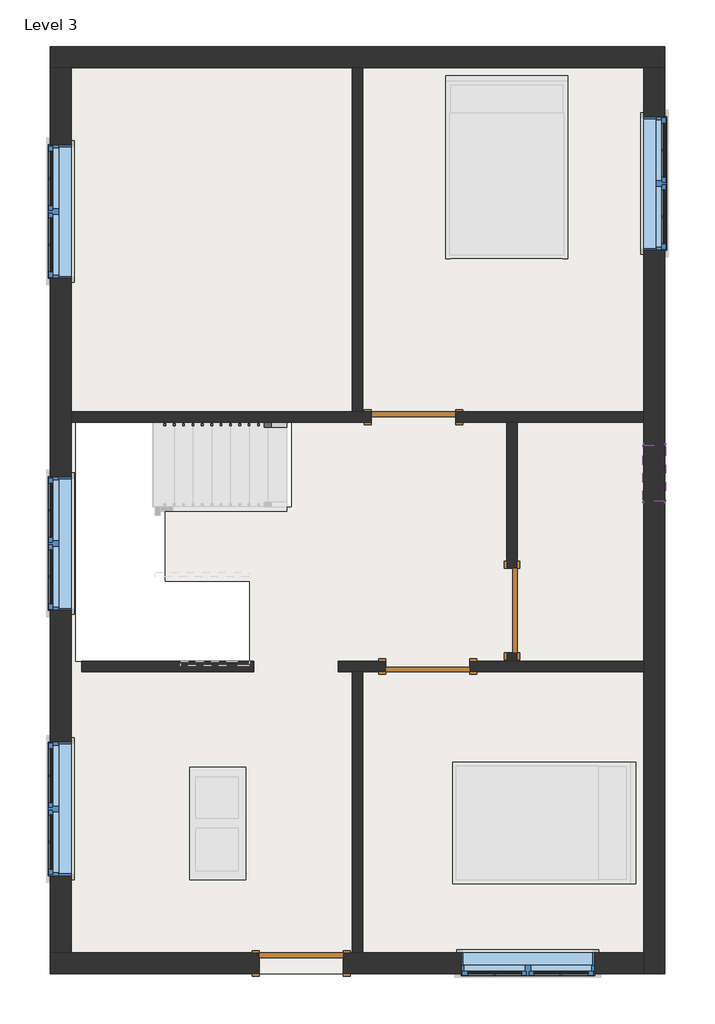
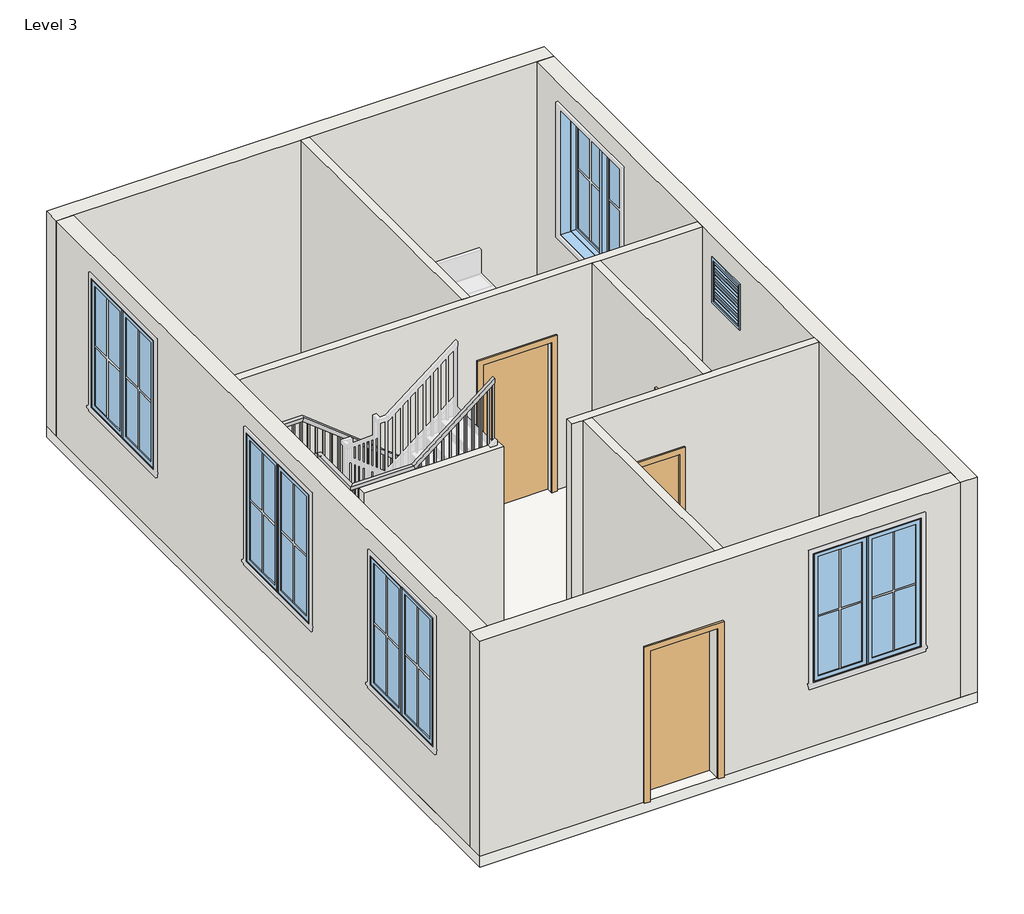
# One storey, part 1 of 2: 10 walls, 6 windows, 4 doors, 1 railing, 1 slab.
"""IFC4 building model written with IfcOpenShell, lengths in millimetres."""

from ifc_helpers import new_model, si_unit, frame, origin, place, context, project, spatial, polyline, outline, extrude, faceted_brep, transform, mapped, element, save
from components import door_e5f9f3c4, door_0ca8825f, window_9ac97e1a, window_f2d8fef0

model = new_model("IFC4")

# Units and contexts
model_context = context("Model", 3, world=origin())
ifc_project = project(units=[si_unit("LENGTHUNIT", "METRE", prefix="MILLI")], contexts=[model_context])

# Site, building, storey
site = spatial("IfcSite", under=ifc_project)
building = spatial("IfcBuilding", under=site)
storey = spatial("IfcBuildingStorey", under=building, Name="Level 3", Elevation=3200.4)

# Doors
placement = place(None, origin())
door_shape = door_e5f9f3c4(model_context)
element("IfcDoor", 1, ObjectType="Single-Flush : 36\" x 84\"", at=placement, inside=storey, context=model_context, shape_type="MappedRepresentation", body=[
    mapped(door_shape, transform((-2225.1840247, 979.1819954, 3200.4), x_axis=(1.0, 0.0, 0.0), y_axis=(0.0, 1.0, 0.0), z_axis=(0.0, 0.0, 1.0))),
])
element("IfcDoor", 2, ObjectType="Single-Flush : 36\" x 84\"", at=placement, inside=storey, context=model_context, shape_type="MappedRepresentation", body=[
    mapped(door_shape, transform((-1158.3840247, -1116.3180046, 3200.4), x_axis=(0.0, -1.0, 0.0), y_axis=(1.0, 0.0, 0.0), z_axis=(0.0, 0.0, 1.0))),
])
element("IfcDoor", 3, ObjectType="Single-Flush : 36\" x 84\"", at=placement, inside=storey, context=model_context, shape_type="MappedRepresentation", body=[
    mapped(door_shape, transform((-2072.7840247, -1725.9180046, 3200.4), x_axis=(-1.0, 0.0, 0.0), y_axis=(0.0, -1.0, 0.0), z_axis=(0.0, 0.0, 1.0))),
])
door_2_shape = door_0ca8825f(model_context)
element("IfcDoor", 4, ObjectType="Single-Flush : 36\" x 84\"", at=placement, inside=storey, context=model_context, shape_type="MappedRepresentation", body=[
    mapped(door_2_shape, transform((-3444.3840247, -4945.3680046, 3200.4), x_axis=(1.0, 0.0, 0.0), y_axis=(0.0, 1.0, 0.0), z_axis=(0.0, 0.0, 1.0))),
])

# Railing
element("IfcRailing", 5, ObjectType="Handrail - Rectangular", at=placement, inside=storey, context=model_context, shape_type="SolidModel", body=[
    faceted_brep([(-3603.1340247, 871.2319954, 4275.2210526), (-3603.1340247, 871.2319954, 4210.4980109), (-3603.1340247, 922.0319954, 4210.4980109), (-3603.1340247, 922.0319954, 4275.2210526), (-5097.5006913, 871.2319954, 5454.9842105), (-5115.1365442, 871.2319954, 5404.1842105), (-5115.1365442, 922.0319954, 5404.1842105), (-5097.5006913, 922.0319954, 5454.9842105), (-5889.1340247, 871.2319954, 5454.9842105), (-5889.1340247, 871.2319954, 5404.1842105), (-5939.9340247, 922.0319954, 5404.1842105), (-5939.9340247, 922.0319954, 5454.9842105), (-5889.1340247, 130.6632454, 5454.9842105), (-5889.1340247, 112.1228815, 5404.1842105), (-5939.9340247, 112.1228815, 5404.1842105), (-5939.9340247, 130.6632454, 5454.9842105), (-5889.1340247, -877.3992546, 6303.8789474), (-5889.1340247, -895.9396185, 6253.0789474), (-5939.9340247, -895.9396185, 6253.0789474), (-5939.9340247, -877.3992546, 6303.8789474), (-5889.1340247, -1617.9680046, 6303.8789474), (-5889.1340247, -1617.9680046, 6253.0789474), (-5939.9340247, -1668.7680046, 6253.0789474), (-5939.9340247, -1668.7680046, 6303.8789474), (-5097.5006913, -1617.9680046, 6303.8789474), (-5079.8648385, -1617.9680046, 6253.0789474), (-5079.8648385, -1668.7680046, 6253.0789474), (-5097.5006913, -1668.7680046, 6303.8789474), (-4009.5340247, -1617.9680046, 7162.8), (-4009.5340247, -1668.7680046, 7162.8), (-4009.5340247, -1668.7680046, 7098.0769583), (-4009.5340247, -1617.9680046, 7098.0769583)], [[[0, 1, 2, 3]], [[1, 0, 4, 5]], [[2, 1, 5, 6]], [[3, 2, 6, 7]], [[0, 3, 7, 4]], [[5, 4, 8, 9]], [[6, 5, 9, 10]], [[7, 6, 10, 11]], [[4, 7, 11, 8]], [[9, 8, 12, 13]], [[10, 9, 13, 14]], [[11, 10, 14, 15]], [[8, 11, 15, 12]], [[13, 12, 16, 17]], [[14, 13, 17, 18]], [[15, 14, 18, 19]], [[12, 15, 19, 16]], [[17, 16, 20, 21]], [[18, 17, 21, 22]], [[19, 18, 22, 23]], [[16, 19, 23, 20]], [[21, 20, 24, 25]], [[22, 21, 25, 26]], [[23, 22, 26, 27]], [[20, 23, 27, 24]], [[28, 29, 30, 31]], [[25, 24, 28, 31]], [[26, 25, 31, 30]], [[27, 26, 30, 29]], [[24, 27, 29, 28]]]),
    extrude(outline(polyline([(7045.4388004, -4076.2090247), (7030.3993267, -4095.2590247), (6087.9789474, -4095.2590247), (6087.9789474, -4076.2090247), (7045.4388004, -4076.2090247)])), frame((0.0, -1652.8930046, 0.0), z_axis=(0.0, 1.0, 0.0), x_axis=(0.0, 0.0, 1.0)), (0.0, 0.0, 1.0), 19.05),
    extrude(outline(polyline([(6965.228274, -4177.8090247), (6950.1888004, -4196.8590247), (6087.9789474, -4196.8590247), (6087.9789474, -4177.8090247), (6965.228274, -4177.8090247)])), frame((0.0, -1652.8930046, 0.0), z_axis=(0.0, 1.0, 0.0), x_axis=(0.0, 0.0, 1.0)), (0.0, 0.0, 1.0), 19.05),
    extrude(outline(polyline([(6885.0177477, -4279.4090247), (6869.978274, -4298.4590247), (5927.5578947, -4298.4590247), (5927.5578947, -4279.4090247), (6885.0177477, -4279.4090247)])), frame((0.0, -1652.8930046, 0.0), z_axis=(0.0, 1.0, 0.0), x_axis=(0.0, 0.0, 1.0)), (0.0, 0.0, 1.0), 19.05),
    extrude(outline(polyline([(6804.8072214, -4381.0090247), (6789.7677477, -4400.0590247), (5927.5578947, -4400.0590247), (5927.5578947, -4381.0090247), (6804.8072214, -4381.0090247)])), frame((0.0, -1652.8930046, 0.0), z_axis=(0.0, 1.0, 0.0), x_axis=(0.0, 0.0, 1.0)), (0.0, 0.0, 1.0), 19.05),
    extrude(outline(polyline([(6724.5966951, -4482.6090247), (6709.5572214, -4501.6590247), (5767.1368421, -4501.6590247), (5767.1368421, -4482.6090247), (6724.5966951, -4482.6090247)])), frame((0.0, -1652.8930046, 0.0), z_axis=(0.0, 1.0, 0.0), x_axis=(0.0, 0.0, 1.0)), (0.0, 0.0, 1.0), 19.05),
    extrude(outline(polyline([(6644.3861688, -4584.2090247), (6629.3466951, -4603.2590247), (5767.1368421, -4603.2590247), (5767.1368421, -4584.2090247), (6644.3861688, -4584.2090247)])), frame((0.0, -1652.8930046, 0.0), z_axis=(0.0, 1.0, 0.0), x_axis=(0.0, 0.0, 1.0)), (0.0, 0.0, 1.0), 19.05),
    extrude(outline(polyline([(6564.1756425, -4685.8090247), (6549.1361688, -4704.8590247), (5606.7157895, -4704.8590247), (5606.7157895, -4685.8090247), (6564.1756425, -4685.8090247)])), frame((0.0, -1652.8930046, 0.0), z_axis=(0.0, 1.0, 0.0), x_axis=(0.0, 0.0, 1.0)), (0.0, 0.0, 1.0), 19.05),
    extrude(outline(polyline([(6483.9651161, -4787.4090247), (6468.9256425, -4806.4590247), (5606.7157895, -4806.4590247), (5606.7157895, -4787.4090247), (6483.9651161, -4787.4090247)])), frame((0.0, -1652.8930046, 0.0), z_axis=(0.0, 1.0, 0.0), x_axis=(0.0, 0.0, 1.0)), (0.0, 0.0, 1.0), 19.05),
    extrude(outline(polyline([(6403.7545898, -4889.0090247), (6388.7151161, -4908.0590247), (5446.2947368, -4908.0590247), (5446.2947368, -4889.0090247), (6403.7545898, -4889.0090247)])), frame((0.0, -1652.8930046, 0.0), z_axis=(0.0, 1.0, 0.0), x_axis=(0.0, 0.0, 1.0)), (0.0, 0.0, 1.0), 19.05),
    extrude(outline(polyline([(6323.5440635, -4990.6090247), (6308.5045898, -5009.6590247), (5446.2947368, -5009.6590247), (5446.2947368, -4990.6090247), (6323.5440635, -4990.6090247)])), frame((0.0, -1652.8930046, 0.0), z_axis=(0.0, 1.0, 0.0), x_axis=(0.0, 0.0, 1.0)), (0.0, 0.0, 1.0), 19.05),
    extrude(outline(polyline([(-5111.2590247, -1652.8930046), (-5111.2590247, -1633.8430046), (-5092.2090247, -1633.8430046), (-5092.2090247, -1652.8930046), (-5111.2590247, -1652.8930046)])), frame((0.0, 0.0, 5285.8736842), z_axis=(0.0, 0.0, 1.0), x_axis=(1.0, 0.0, 0.0)), (0.0, 0.0, 1.0), 967.2052632),
    extrude(outline(polyline([(-5212.8590247, -1652.8930046), (-5212.8590247, -1633.8430046), (-5193.8090247, -1633.8430046), (-5193.8090247, -1652.8930046), (-5212.8590247, -1652.8930046)])), frame((0.0, 0.0, 5285.8736842), z_axis=(0.0, 0.0, 1.0), x_axis=(1.0, 0.0, 0.0)), (0.0, 0.0, 1.0), 967.2052632),
    extrude(outline(polyline([(-5314.4590247, -1652.8930046), (-5314.4590247, -1633.8430046), (-5295.4090247, -1633.8430046), (-5295.4090247, -1652.8930046), (-5314.4590247, -1652.8930046)])), frame((0.0, 0.0, 5285.8736842), z_axis=(0.0, 0.0, 1.0), x_axis=(1.0, 0.0, 0.0)), (0.0, 0.0, 1.0), 967.2052632),
    extrude(outline(polyline([(-5416.0590247, -1652.8930046), (-5416.0590247, -1633.8430046), (-5397.0090247, -1633.8430046), (-5397.0090247, -1652.8930046), (-5416.0590247, -1652.8930046)])), frame((0.0, 0.0, 5285.8736842), z_axis=(0.0, 0.0, 1.0), x_axis=(1.0, 0.0, 0.0)), (0.0, 0.0, 1.0), 967.2052632),
    extrude(outline(polyline([(-5517.6590247, -1652.8930046), (-5517.6590247, -1633.8430046), (-5498.6090247, -1633.8430046), (-5498.6090247, -1652.8930046), (-5517.6590247, -1652.8930046)])), frame((0.0, 0.0, 5285.8736842), z_axis=(0.0, 0.0, 1.0), x_axis=(1.0, 0.0, 0.0)), (0.0, 0.0, 1.0), 967.2052632),
    extrude(outline(polyline([(-5619.2590247, -1652.8930046), (-5619.2590247, -1633.8430046), (-5600.2090247, -1633.8430046), (-5600.2090247, -1652.8930046), (-5619.2590247, -1652.8930046)])), frame((0.0, 0.0, 5285.8736842), z_axis=(0.0, 0.0, 1.0), x_axis=(1.0, 0.0, 0.0)), (0.0, 0.0, 1.0), 967.2052632),
    extrude(outline(polyline([(-5720.8590247, -1652.8930046), (-5720.8590247, -1633.8430046), (-5701.8090247, -1633.8430046), (-5701.8090247, -1652.8930046), (-5720.8590247, -1652.8930046)])), frame((0.0, 0.0, 5285.8736842), z_axis=(0.0, 0.0, 1.0), x_axis=(1.0, 0.0, 0.0)), (0.0, 0.0, 1.0), 967.2052632),
    extrude(outline(polyline([(-5822.4590247, -1652.8930046), (-5822.4590247, -1633.8430046), (-5803.4090247, -1633.8430046), (-5803.4090247, -1652.8930046), (-5822.4590247, -1652.8930046)])), frame((0.0, 0.0, 5285.8736842), z_axis=(0.0, 0.0, 1.0), x_axis=(1.0, 0.0, 0.0)), (0.0, 0.0, 1.0), 967.2052632),
    extrude(outline(polyline([(-5924.0590247, -1532.2430046), (-5905.0090247, -1532.2430046), (-5905.0090247, -1551.2930046), (-5924.0590247, -1551.2930046), (-5924.0590247, -1532.2430046)])), frame((0.0, 0.0, 5285.8736842), z_axis=(0.0, 0.0, 1.0), x_axis=(1.0, 0.0, 0.0)), (0.0, 0.0, 1.0), 967.2052632),
    extrude(outline(polyline([(-5924.0590247, -1430.6430046), (-5905.0090247, -1430.6430046), (-5905.0090247, -1449.6930046), (-5924.0590247, -1449.6930046), (-5924.0590247, -1430.6430046)])), frame((0.0, 0.0, 5285.8736842), z_axis=(0.0, 0.0, 1.0), x_axis=(1.0, 0.0, 0.0)), (0.0, 0.0, 1.0), 967.2052632),
    extrude(outline(polyline([(-5924.0590247, -1329.0430046), (-5905.0090247, -1329.0430046), (-5905.0090247, -1348.0930046), (-5924.0590247, -1348.0930046), (-5924.0590247, -1329.0430046)])), frame((0.0, 0.0, 5285.8736842), z_axis=(0.0, 0.0, 1.0), x_axis=(1.0, 0.0, 0.0)), (0.0, 0.0, 1.0), 967.2052632),
    extrude(outline(polyline([(-5924.0590247, -1227.4430046), (-5905.0090247, -1227.4430046), (-5905.0090247, -1246.4930046), (-5924.0590247, -1246.4930046), (-5924.0590247, -1227.4430046)])), frame((0.0, 0.0, 5285.8736842), z_axis=(0.0, 0.0, 1.0), x_axis=(1.0, 0.0, 0.0)), (0.0, 0.0, 1.0), 967.2052632),
    extrude(outline(polyline([(-5924.0590247, -1125.8430046), (-5905.0090247, -1125.8430046), (-5905.0090247, -1144.8930046), (-5924.0590247, -1144.8930046), (-5924.0590247, -1125.8430046)])), frame((0.0, 0.0, 5285.8736842), z_axis=(0.0, 0.0, 1.0), x_axis=(1.0, 0.0, 0.0)), (0.0, 0.0, 1.0), 967.2052632),
    extrude(outline(polyline([(-5924.0590247, -1024.2430046), (-5905.0090247, -1024.2430046), (-5905.0090247, -1043.2930046), (-5924.0590247, -1043.2930046), (-5924.0590247, -1024.2430046)])), frame((0.0, 0.0, 5285.8736842), z_axis=(0.0, 0.0, 1.0), x_axis=(1.0, 0.0, 0.0)), (0.0, 0.0, 1.0), 967.2052632),
    extrude(outline(polyline([(-5924.0590247, -922.6430046), (-5905.0090247, -922.6430046), (-5905.0090247, -941.6930046), (-5924.0590247, -941.6930046), (-5924.0590247, -922.6430046)])), frame((0.0, 0.0, 5285.8736842), z_axis=(0.0, 0.0, 1.0), x_axis=(1.0, 0.0, 0.0)), (0.0, 0.0, 1.0), 967.2052632),
    extrude(outline(polyline([(-840.0930046, 6206.0502199), (-821.0430046, 6190.0081146), (-821.0430046, 5285.8736842), (-840.0930046, 5285.8736842), (-840.0930046, 6206.0502199)])), frame((-5924.0590247, 0.0, 0.0), z_axis=(1.0, 0.0, 0.0), x_axis=(0.0, 1.0, 0.0)), (0.0, 0.0, 1.0), 19.05),
    extrude(outline(polyline([(-738.4930046, 6120.4923251), (-719.4430046, 6104.4502199), (-719.4430046, 5125.4526316), (-738.4930046, 5125.4526316), (-738.4930046, 6120.4923251)])), frame((-5924.0590247, 0.0, 0.0), z_axis=(1.0, 0.0, 0.0), x_axis=(0.0, 1.0, 0.0)), (0.0, 0.0, 1.0), 19.05),
    extrude(outline(polyline([(-636.8930046, 6034.9344304), (-617.8430046, 6018.8923251), (-617.8430046, 5125.4526316), (-636.8930046, 5125.4526316), (-636.8930046, 6034.9344304)])), frame((-5924.0590247, 0.0, 0.0), z_axis=(1.0, 0.0, 0.0), x_axis=(0.0, 1.0, 0.0)), (0.0, 0.0, 1.0), 19.05),
    extrude(outline(polyline([(-535.2930046, 5949.3765357), (-516.2430046, 5933.3344304), (-516.2430046, 4965.0315789), (-535.2930046, 4965.0315789), (-535.2930046, 5949.3765357)])), frame((-5924.0590247, 0.0, 0.0), z_axis=(1.0, 0.0, 0.0), x_axis=(0.0, 1.0, 0.0)), (0.0, 0.0, 1.0), 19.05),
    extrude(outline(polyline([(-433.6930046, 5863.8186409), (-414.6430046, 5847.7765357), (-414.6430046, 4965.0315789), (-433.6930046, 4965.0315789), (-433.6930046, 5863.8186409)])), frame((-5924.0590247, 0.0, 0.0), z_axis=(1.0, 0.0, 0.0), x_axis=(0.0, 1.0, 0.0)), (0.0, 0.0, 1.0), 19.05),
    extrude(outline(polyline([(-332.0930046, 5778.2607462), (-313.0430046, 5762.2186409), (-313.0430046, 4804.6105263), (-332.0930046, 4804.6105263), (-332.0930046, 5778.2607462)])), frame((-5924.0590247, 0.0, 0.0), z_axis=(1.0, 0.0, 0.0), x_axis=(0.0, 1.0, 0.0)), (0.0, 0.0, 1.0), 19.05),
    extrude(outline(polyline([(-230.4930046, 5692.7028514), (-211.4430046, 5676.6607462), (-211.4430046, 4804.6105263), (-230.4930046, 4804.6105263), (-230.4930046, 5692.7028514)])), frame((-5924.0590247, 0.0, 0.0), z_axis=(1.0, 0.0, 0.0), x_axis=(0.0, 1.0, 0.0)), (0.0, 0.0, 1.0), 19.05),
    extrude(outline(polyline([(-128.8930046, 5607.1449567), (-109.8430046, 5591.1028514), (-109.8430046, 4644.1894737), (-128.8930046, 4644.1894737), (-128.8930046, 5607.1449567)])), frame((-5924.0590247, 0.0, 0.0), z_axis=(1.0, 0.0, 0.0), x_axis=(0.0, 1.0, 0.0)), (0.0, 0.0, 1.0), 19.05),
    extrude(outline(polyline([(-27.2930046, 5521.587062), (-8.2430046, 5505.5449567), (-8.2430046, 4644.1894737), (-27.2930046, 4644.1894737), (-27.2930046, 5521.587062)])), frame((-5924.0590247, 0.0, 0.0), z_axis=(1.0, 0.0, 0.0), x_axis=(0.0, 1.0, 0.0)), (0.0, 0.0, 1.0), 19.05),
    extrude(outline(polyline([(74.3069954, 5436.0291672), (93.3569954, 5419.987062), (93.3569954, 4483.7684211), (74.3069954, 4483.7684211), (74.3069954, 5436.0291672)])), frame((-5924.0590247, 0.0, 0.0), z_axis=(1.0, 0.0, 0.0), x_axis=(0.0, 1.0, 0.0)), (0.0, 0.0, 1.0), 19.05),
    extrude(outline(polyline([(-5924.0590247, 194.9569954), (-5905.0090247, 194.9569954), (-5905.0090247, 175.9069954), (-5924.0590247, 175.9069954), (-5924.0590247, 194.9569954)])), frame((0.0, 0.0, 4483.7684211), z_axis=(0.0, 0.0, 1.0), x_axis=(1.0, 0.0, 0.0)), (0.0, 0.0, 1.0), 920.4157895),
    extrude(outline(polyline([(-5924.0590247, 296.5569954), (-5905.0090247, 296.5569954), (-5905.0090247, 277.5069954), (-5924.0590247, 277.5069954), (-5924.0590247, 296.5569954)])), frame((0.0, 0.0, 4483.7684211), z_axis=(0.0, 0.0, 1.0), x_axis=(1.0, 0.0, 0.0)), (0.0, 0.0, 1.0), 920.4157895),
    extrude(outline(polyline([(-5924.0590247, 398.1569954), (-5905.0090247, 398.1569954), (-5905.0090247, 379.1069954), (-5924.0590247, 379.1069954), (-5924.0590247, 398.1569954)])), frame((0.0, 0.0, 4483.7684211), z_axis=(0.0, 0.0, 1.0), x_axis=(1.0, 0.0, 0.0)), (0.0, 0.0, 1.0), 920.4157895),
    extrude(outline(polyline([(-5924.0590247, 499.7569954), (-5905.0090247, 499.7569954), (-5905.0090247, 480.7069954), (-5924.0590247, 480.7069954), (-5924.0590247, 499.7569954)])), frame((0.0, 0.0, 4483.7684211), z_axis=(0.0, 0.0, 1.0), x_axis=(1.0, 0.0, 0.0)), (0.0, 0.0, 1.0), 920.4157895),
    extrude(outline(polyline([(-5924.0590247, 601.3569954), (-5905.0090247, 601.3569954), (-5905.0090247, 582.3069954), (-5924.0590247, 582.3069954), (-5924.0590247, 601.3569954)])), frame((0.0, 0.0, 4483.7684211), z_axis=(0.0, 0.0, 1.0), x_axis=(1.0, 0.0, 0.0)), (0.0, 0.0, 1.0), 920.4157895),
    extrude(outline(polyline([(-5924.0590247, 702.9569954), (-5905.0090247, 702.9569954), (-5905.0090247, 683.9069954), (-5924.0590247, 683.9069954), (-5924.0590247, 702.9569954)])), frame((0.0, 0.0, 4483.7684211), z_axis=(0.0, 0.0, 1.0), x_axis=(1.0, 0.0, 0.0)), (0.0, 0.0, 1.0), 920.4157895),
    extrude(outline(polyline([(-5924.0590247, 804.5569954), (-5905.0090247, 804.5569954), (-5905.0090247, 785.5069954), (-5924.0590247, 785.5069954), (-5924.0590247, 804.5569954)])), frame((0.0, 0.0, 4483.7684211), z_axis=(0.0, 0.0, 1.0), x_axis=(1.0, 0.0, 0.0)), (0.0, 0.0, 1.0), 920.4157895),
    extrude(outline(polyline([(-5828.8090247, 906.1569954), (-5828.8090247, 887.1069954), (-5847.8590247, 887.1069954), (-5847.8590247, 906.1569954), (-5828.8090247, 906.1569954)])), frame((0.0, 0.0, 4483.7684211), z_axis=(0.0, 0.0, 1.0), x_axis=(1.0, 0.0, 0.0)), (0.0, 0.0, 1.0), 920.4157895),
    extrude(outline(polyline([(-5727.2090247, 906.1569954), (-5727.2090247, 887.1069954), (-5746.2590247, 887.1069954), (-5746.2590247, 906.1569954), (-5727.2090247, 906.1569954)])), frame((0.0, 0.0, 4483.7684211), z_axis=(0.0, 0.0, 1.0), x_axis=(1.0, 0.0, 0.0)), (0.0, 0.0, 1.0), 920.4157895),
    extrude(outline(polyline([(-5625.6090247, 906.1569954), (-5625.6090247, 887.1069954), (-5644.6590247, 887.1069954), (-5644.6590247, 906.1569954), (-5625.6090247, 906.1569954)])), frame((0.0, 0.0, 4483.7684211), z_axis=(0.0, 0.0, 1.0), x_axis=(1.0, 0.0, 0.0)), (0.0, 0.0, 1.0), 920.4157895),
    extrude(outline(polyline([(-5524.0090247, 906.1569954), (-5524.0090247, 887.1069954), (-5543.0590247, 887.1069954), (-5543.0590247, 906.1569954), (-5524.0090247, 906.1569954)])), frame((0.0, 0.0, 4483.7684211), z_axis=(0.0, 0.0, 1.0), x_axis=(1.0, 0.0, 0.0)), (0.0, 0.0, 1.0), 920.4157895),
    extrude(outline(polyline([(-5422.4090247, 906.1569954), (-5422.4090247, 887.1069954), (-5441.4590247, 887.1069954), (-5441.4590247, 906.1569954), (-5422.4090247, 906.1569954)])), frame((0.0, 0.0, 4483.7684211), z_axis=(0.0, 0.0, 1.0), x_axis=(1.0, 0.0, 0.0)), (0.0, 0.0, 1.0), 920.4157895),
    extrude(outline(polyline([(-5320.8090247, 906.1569954), (-5320.8090247, 887.1069954), (-5339.8590247, 887.1069954), (-5339.8590247, 906.1569954), (-5320.8090247, 906.1569954)])), frame((0.0, 0.0, 4483.7684211), z_axis=(0.0, 0.0, 1.0), x_axis=(1.0, 0.0, 0.0)), (0.0, 0.0, 1.0), 920.4157895),
    extrude(outline(polyline([(-5219.2090247, 906.1569954), (-5219.2090247, 887.1069954), (-5238.2590247, 887.1069954), (-5238.2590247, 906.1569954), (-5219.2090247, 906.1569954)])), frame((0.0, 0.0, 4483.7684211), z_axis=(0.0, 0.0, 1.0), x_axis=(1.0, 0.0, 0.0)), (0.0, 0.0, 1.0), 920.4157895),
    extrude(outline(polyline([(-5117.6090247, 906.1569954), (-5117.6090247, 887.1069954), (-5136.6590247, 887.1069954), (-5136.6590247, 906.1569954), (-5117.6090247, 906.1569954)])), frame((0.0, 0.0, 4483.7684211), z_axis=(0.0, 0.0, 1.0), x_axis=(1.0, 0.0, 0.0)), (0.0, 0.0, 1.0), 920.4157895),
    extrude(outline(polyline([(5325.9256425, -5016.0090247), (5340.9651161, -5035.0590247), (4483.7684211, -5035.0590247), (4483.7684211, -5016.0090247), (5325.9256425, -5016.0090247)])), frame((0.0, 887.1069954, 0.0), z_axis=(0.0, 1.0, 0.0), x_axis=(0.0, 0.0, 1.0)), (0.0, 0.0, 1.0), 19.05),
    extrude(outline(polyline([(5245.7151161, -4914.4090247), (5260.7545898, -4933.4590247), (4323.3473684, -4933.4590247), (4323.3473684, -4914.4090247), (5245.7151161, -4914.4090247)])), frame((0.0, 887.1069954, 0.0), z_axis=(0.0, 1.0, 0.0), x_axis=(0.0, 0.0, 1.0)), (0.0, 0.0, 1.0), 19.05),
    extrude(outline(polyline([(5165.5045898, -4812.8090247), (5180.5440635, -4831.8590247), (4323.3473684, -4831.8590247), (4323.3473684, -4812.8090247), (5165.5045898, -4812.8090247)])), frame((0.0, 887.1069954, 0.0), z_axis=(0.0, 1.0, 0.0), x_axis=(0.0, 0.0, 1.0)), (0.0, 0.0, 1.0), 19.05),
    extrude(outline(polyline([(5085.2940635, -4711.2090247), (5100.3335372, -4730.2590247), (4162.9263158, -4730.2590247), (4162.9263158, -4711.2090247), (5085.2940635, -4711.2090247)])), frame((0.0, 887.1069954, 0.0), z_axis=(0.0, 1.0, 0.0), x_axis=(0.0, 0.0, 1.0)), (0.0, 0.0, 1.0), 19.05),
    extrude(outline(polyline([(5005.0835372, -4609.6090247), (5020.1230109, -4628.6590247), (4162.9263158, -4628.6590247), (4162.9263158, -4609.6090247), (5005.0835372, -4609.6090247)])), frame((0.0, 887.1069954, 0.0), z_axis=(0.0, 1.0, 0.0), x_axis=(0.0, 0.0, 1.0)), (0.0, 0.0, 1.0), 19.05),
    extrude(outline(polyline([(4924.8730109, -4508.0090247), (4939.9124846, -4527.0590247), (4002.5052632, -4527.0590247), (4002.5052632, -4508.0090247), (4924.8730109, -4508.0090247)])), frame((0.0, 887.1069954, 0.0), z_axis=(0.0, 1.0, 0.0), x_axis=(0.0, 0.0, 1.0)), (0.0, 0.0, 1.0), 19.05),
    extrude(outline(polyline([(4844.6624846, -4406.4090247), (4859.7019583, -4425.4590247), (4002.5052632, -4425.4590247), (4002.5052632, -4406.4090247), (4844.6624846, -4406.4090247)])), frame((0.0, 887.1069954, 0.0), z_axis=(0.0, 1.0, 0.0), x_axis=(0.0, 0.0, 1.0)), (0.0, 0.0, 1.0), 19.05),
    extrude(outline(polyline([(4764.4519583, -4304.8090247), (4779.4914319, -4323.8590247), (3842.0842105, -4323.8590247), (3842.0842105, -4304.8090247), (4764.4519583, -4304.8090247)])), frame((0.0, 887.1069954, 0.0), z_axis=(0.0, 1.0, 0.0), x_axis=(0.0, 0.0, 1.0)), (0.0, 0.0, 1.0), 19.05),
    extrude(outline(polyline([(4684.2414319, -4203.2090247), (4699.2809056, -4222.2590247), (3842.0842105, -4222.2590247), (3842.0842105, -4203.2090247), (4684.2414319, -4203.2090247)])), frame((0.0, 887.1069954, 0.0), z_axis=(0.0, 1.0, 0.0), x_axis=(0.0, 0.0, 1.0)), (0.0, 0.0, 1.0), 19.05),
    extrude(outline(polyline([(4604.0309056, -4101.6090247), (4619.0703793, -4120.6590247), (3681.6631579, -4120.6590247), (3681.6631579, -4101.6090247), (4604.0309056, -4101.6090247)])), frame((0.0, 887.1069954, 0.0), z_axis=(0.0, 1.0, 0.0), x_axis=(0.0, 0.0, 1.0)), (0.0, 0.0, 1.0), 19.05),
    extrude(outline(polyline([(4523.8203793, -4000.0090247), (4538.859853, -4019.0590247), (3681.6631579, -4019.0590247), (3681.6631579, -4000.0090247), (4523.8203793, -4000.0090247)])), frame((0.0, 887.1069954, 0.0), z_axis=(0.0, 1.0, 0.0), x_axis=(0.0, 0.0, 1.0)), (0.0, 0.0, 1.0), 19.05),
    extrude(outline(polyline([(4443.609853, -3898.4090247), (4458.6493267, -3917.4590247), (3521.2421053, -3917.4590247), (3521.2421053, -3898.4090247), (4443.609853, -3898.4090247)])), frame((0.0, 887.1069954, 0.0), z_axis=(0.0, 1.0, 0.0), x_axis=(0.0, 0.0, 1.0)), (0.0, 0.0, 1.0), 19.05),
    extrude(outline(polyline([(4363.3993267, -3796.8090247), (4378.4388004, -3815.8590247), (3521.2421053, -3815.8590247), (3521.2421053, -3796.8090247), (4363.3993267, -3796.8090247)])), frame((0.0, 887.1069954, 0.0), z_axis=(0.0, 1.0, 0.0), x_axis=(0.0, 0.0, 1.0)), (0.0, 0.0, 1.0), 19.05),
    extrude(outline(polyline([(4283.1888004, -3695.2090247), (4298.228274, -3714.2590247), (3360.8210526, -3714.2590247), (3360.8210526, -3695.2090247), (4283.1888004, -3695.2090247)])), frame((0.0, 887.1069954, 0.0), z_axis=(0.0, 1.0, 0.0), x_axis=(0.0, 0.0, 1.0)), (0.0, 0.0, 1.0), 19.05),
    extrude(outline(polyline([(-5924.0590247, -1633.8430046), (-5905.0090247, -1633.8430046), (-5905.0090247, -1652.8930046), (-5924.0590247, -1652.8930046), (-5924.0590247, -1633.8430046)])), frame((0.0, 0.0, 5285.8736842), z_axis=(0.0, 0.0, 1.0), x_axis=(1.0, 0.0, 0.0)), (0.0, 0.0, 1.0), 967.2052632),
    extrude(outline(polyline([(-5905.0090247, 906.1569954), (-5905.0090247, 887.1069954), (-5924.0590247, 887.1069954), (-5924.0590247, 906.1569954), (-5905.0090247, 906.1569954)])), frame((0.0, 0.0, 4483.7684211), z_axis=(0.0, 0.0, 1.0), x_axis=(1.0, 0.0, 0.0)), (0.0, 0.0, 1.0), 920.4157895),
    extrude(outline(polyline([(7098.0769583, -4009.5340247), (7083.0374846, -4028.5840247), (6087.9789474, -4028.5840247), (6087.9789474, -4009.5340247), (7098.0769583, -4009.5340247)])), frame((0.0, -1652.8930046, 0.0), z_axis=(0.0, 1.0, 0.0), x_axis=(0.0, 0.0, 1.0)), (0.0, 0.0, 1.0), 19.05),
    extrude(outline(polyline([(4210.4980109, -3603.1340247), (4225.5374846, -3622.1840247), (3360.8210526, -3622.1840247), (3360.8210526, -3603.1340247), (4210.4980109, -3603.1340247)])), frame((0.0, 887.1069954, 0.0), z_axis=(0.0, 1.0, 0.0), x_axis=(0.0, 0.0, 1.0)), (0.0, 0.0, 1.0), 19.05),
])

# Slab
element("IfcSlab", 6, ObjectType="FLOOR 6\"", at=placement, inside=storey, context=model_context, shape_type="SweptSolid", body=[
    extrude(outline(polyline([(498.9659753, 4998.7319954), (498.9659753, -5059.6680046), (-6168.5340247, -5059.6680046), (-6168.5340247, 4998.7319954), (498.9659753, 4998.7319954)]), holes=[polyline([(-5889.1340247, 922.0319954), (-5889.1340247, -1668.7680046), (-4009.5340247, -1668.7680046), (-4009.5340247, -805.1680046), (-4923.9340247, -805.1680046), (-4923.9340247, 7.6319954), (-3552.3340247, 7.6319954), (-3552.3340247, 922.0319954), (-5889.1340247, 922.0319954)])]), frame((0.0, 0.0, 3048.0), z_axis=(0.0, 0.0, 1.0), x_axis=(1.0, 0.0, 0.0)), (0.0, 0.0, 1.0), 152.4),
])

# Walls
element("IfcWall", 7, ObjectType="WALL 4.5\"", at=placement, inside=storey, context=model_context, shape_type="SweptSolid", body=[
    extrude(outline(polyline([(-2891.9340247, 1036.3319954), (-2891.9340247, 4770.1319954), (-2777.6340247, 4770.1319954), (-2777.6340247, 1036.3319954), (-2891.9340247, 1036.3319954)])), frame((0.0, 0.0, 3200.4), z_axis=(0.0, 0.0, 1.0), x_axis=(1.0, 0.0, 0.0)), (0.0, 0.0, 1.0), 3048.0),
])
element("IfcWall", 8, ObjectType="WALL 4.5\"", at=placement, inside=storey, context=model_context, shape_type="Brep", body=[
    faceted_brep([(-1767.9840247, 922.0319954, 5334.0), (-1767.9840247, 922.0319954, 3200.4), (-1215.5340247, 922.0319954, 3200.4), (-1101.2340247, 922.0319954, 3200.4), (270.3659753, 922.0319954, 3200.4), (270.3659753, 922.0319954, 6248.4), (-1101.2340247, 922.0319954, 6248.4), (-1215.5340247, 922.0319954, 6248.4), (-3552.3340247, 922.0319954, 6248.4), (-5889.1340247, 922.0319954, 6248.4), (-5939.9340247, 922.0319954, 6248.4), (-5939.9340247, 922.0319954, 3200.4), (-2682.3840247, 922.0319954, 3200.4), (-2682.3840247, 922.0319954, 5334.0), (270.3659753, 1036.3319954, 3200.4), (-1767.9840247, 1036.3319954, 3200.4), (-1767.9840247, 1036.3319954, 5334.0), (-2682.3840247, 1036.3319954, 5334.0), (-2682.3840247, 1036.3319954, 3200.4), (-2777.6340247, 1036.3319954, 3200.4), (-2891.9340247, 1036.3319954, 3200.4), (-5939.9340247, 1036.3319954, 3200.4), (-5939.9340247, 1036.3319954, 6248.4), (-2891.9340247, 1036.3319954, 6248.4), (-2777.6340247, 1036.3319954, 6248.4), (270.3659753, 1036.3319954, 6248.4)], [[[0, 1, 2, 3, 4, 5, 6, 7, 8, 9, 10, 11, 12, 13]], [[14, 15, 16, 17, 18, 19, 20, 21, 22, 23, 24, 25]], [[12, 11, 21, 20, 19, 18]], [[4, 3, 2, 1, 15, 14]], [[5, 4, 14, 25]], [[11, 10, 22, 21]], [[16, 15, 1, 0]], [[17, 16, 0, 13]], [[18, 17, 13, 12]], [[10, 9, 8, 7, 6, 5, 25, 24, 23, 22]]]),
])
element("IfcWall", 9, ObjectType="WALL 4.5\"", at=placement, inside=storey, context=model_context, shape_type="SweptSolid", body=[
    extrude(outline(polyline([(-1573.5180046, 5334.0), (-1573.5180046, 3200.4), (-1668.7680046, 3200.4), (-1668.7680046, 6248.4), (922.0319954, 6248.4), (922.0319954, 3200.4), (-659.1180046, 3200.4), (-659.1180046, 5334.0), (-1573.5180046, 5334.0)])), frame((-1215.5340247, 0.0, 0.0), z_axis=(1.0, 0.0, 0.0), x_axis=(0.0, 1.0, 0.0)), (0.0, 0.0, 1.0), 114.3),
])
element("IfcWall", 10, ObjectType="WALL 4.5\"", at=placement, inside=storey, context=model_context, shape_type="Brep", body=[
    faceted_brep([(-2529.9840247, -1668.7680046, 5334.0), (-2529.9840247, -1668.7680046, 3200.4), (-3044.3340247, -1668.7680046, 3200.4), (-3044.3340247, -1668.7680046, 6248.4), (-1215.5340247, -1668.7680046, 6248.4), (-1101.2340247, -1668.7680046, 6248.4), (270.3659753, -1668.7680046, 6248.4), (270.3659753, -1668.7680046, 3200.4), (-1101.2340247, -1668.7680046, 3200.4), (-1215.5340247, -1668.7680046, 3200.4), (-1615.5840247, -1668.7680046, 3200.4), (-1615.5840247, -1668.7680046, 5334.0), (-3044.3340247, -1783.0680046, 3200.4), (-2891.9340247, -1783.0680046, 3200.4), (-2777.6340247, -1783.0680046, 3200.4), (-2529.9840247, -1783.0680046, 3200.4), (-2529.9840247, -1783.0680046, 5334.0), (-1615.5840247, -1783.0680046, 5334.0), (-1615.5840247, -1783.0680046, 3200.4), (270.3659753, -1783.0680046, 3200.4), (270.3659753, -1783.0680046, 6248.4), (-2777.6340247, -1783.0680046, 6248.4), (-2891.9340247, -1783.0680046, 6248.4), (-3044.3340247, -1783.0680046, 6248.4)], [[[0, 1, 2, 3, 4, 5, 6, 7, 8, 9, 10, 11]], [[12, 13, 14, 15, 16, 17, 18, 19, 20, 21, 22, 23]], [[2, 1, 15, 14, 13, 12]], [[10, 9, 8, 7, 19, 18]], [[3, 2, 12, 23]], [[7, 6, 20, 19]], [[16, 15, 1, 0]], [[17, 16, 0, 11]], [[18, 17, 11, 10]], [[6, 5, 4, 3, 23, 22, 21, 20]]]),
])
element("IfcWall", 11, ObjectType="WALL 4.5\"", at=placement, inside=storey, context=model_context, shape_type="Brep", body=[
    faceted_brep([(-5825.6340247, -1783.0680046, 3200.4), (-3958.7340247, -1783.0680046, 3200.4), (-3958.7340247, -1783.0680046, 6248.4), (-5825.6340247, -1783.0680046, 6248.4), (-5825.6340247, -1668.7680046, 3200.4), (-5825.6340247, -1668.7680046, 6248.4), (-4009.5340247, -1668.7680046, 6248.4), (-3958.7340247, -1668.7680046, 6248.4), (-3958.7340247, -1668.7680046, 3200.4)], [[[0, 1, 2, 3]], [[4, 5, 6, 7, 8]], [[1, 0, 4, 8]], [[2, 1, 8, 7]], [[0, 3, 5, 4]], [[3, 2, 7, 6, 5]]]),
])
element("IfcWall", 12, ObjectType="WALL 4.5\"", at=placement, inside=storey, context=model_context, shape_type="SweptSolid", body=[
    extrude(outline(polyline([(-2891.9340247, -4831.0680046), (-2891.9340247, -1783.0680046), (-2777.6340247, -1783.0680046), (-2777.6340247, -4831.0680046), (-2891.9340247, -4831.0680046)])), frame((0.0, 0.0, 3200.4), z_axis=(0.0, 0.0, 1.0), x_axis=(1.0, 0.0, 0.0)), (0.0, 0.0, 1.0), 3048.0),
])
element("IfcWall", 13, ObjectType="WALL 9\"", at=placement, inside=storey, context=model_context, shape_type="Brep", body=[
    faceted_brep([(-6168.5340247, 4770.1319954, 3200.4), (-5939.9340247, 4770.1319954, 3200.4), (-2891.9340247, 4770.1319954, 3200.4), (-2777.6340247, 4770.1319954, 3200.4), (270.3659753, 4770.1319954, 3200.4), (498.9659753, 4770.1319954, 3200.4), (498.9659753, 4770.1319954, 6248.4), (270.3659753, 4770.1319954, 6248.4), (-2777.6340247, 4770.1319954, 6248.4), (-2891.9340247, 4770.1319954, 6248.4), (-5939.9340247, 4770.1319954, 6248.4), (-6168.5340247, 4770.1319954, 6248.4), (-6168.5340247, 4998.7319954, 3200.4), (-6168.5340247, 4998.7319954, 6248.4), (498.9659753, 4998.7319954, 6248.4), (498.9659753, 4998.7319954, 3200.4)], [[[0, 1, 2, 3, 4, 5, 6, 7, 8, 9, 10, 11]], [[12, 13, 14, 15]], [[5, 4, 3, 2, 1, 0, 12, 15]], [[6, 5, 15, 14]], [[0, 11, 13, 12]], [[11, 10, 9, 8, 7, 6, 14, 13]]]),
])
element("IfcWall", 14, ObjectType="WALL 9\"", at=placement, inside=storey, context=model_context, shape_type="Brep", body=[
    faceted_brep([(270.3659753, 4770.1319954, 3200.4), (270.3659753, 1036.3319954, 3200.4), (270.3659753, 922.0319954, 3200.4), (270.3659753, -1668.7680046, 3200.4), (270.3659753, -1783.0680046, 3200.4), (270.3659753, -4831.0680046, 3200.4), (270.3659753, -5059.6680046, 3200.4), (270.3659753, -5059.6680046, 6248.4), (270.3659753, -4831.0680046, 6248.4), (270.3659753, -1783.0680046, 6248.4), (270.3659753, -1668.7680046, 6248.4), (270.3659753, 922.0319954, 6248.4), (270.3659753, 1036.3319954, 6248.4), (270.3659753, 4770.1319954, 6248.4), (270.3659753, 2788.9319954, 5943.6), (270.3659753, 2788.9319954, 4114.8), (270.3659753, 4236.7319954, 4114.8), (270.3659753, 4236.7319954, 5943.6), (270.3659753, 64.7819954, 5943.6), (270.3659753, 64.7819954, 5334.0), (270.3659753, 674.3819954, 5334.0), (270.3659753, 674.3819954, 5943.6), (498.9659753, 4770.1319954, 3200.4), (498.9659753, 4770.1319954, 6248.4), (498.9659753, -5059.6680046, 6248.4), (498.9659753, -5059.6680046, 3200.4), (498.9659753, 2788.9319954, 5943.6), (498.9659753, 4236.7319954, 5943.6), (498.9659753, 4236.7319954, 4114.8), (498.9659753, 2788.9319954, 4114.8), (498.9659753, 64.7819954, 5943.6), (498.9659753, 674.3819954, 5943.6), (498.9659753, 674.3819954, 5334.0), (498.9659753, 64.7819954, 5334.0)], [[[0, 1, 2, 3, 4, 5, 6, 7, 8, 9, 10, 11, 12, 13], [14, 15, 16, 17], [18, 19, 20, 21]], [[22, 23, 24, 25], [26, 27, 28, 29], [30, 31, 32, 33]], [[6, 5, 4, 3, 2, 1, 0, 22, 25]], [[0, 13, 23, 22]], [[7, 6, 25, 24]], [[15, 14, 26, 29]], [[16, 15, 29, 28]], [[17, 16, 28, 27]], [[14, 17, 27, 26]], [[19, 18, 30, 33]], [[20, 19, 33, 32]], [[21, 20, 32, 31]], [[18, 21, 31, 30]], [[13, 12, 11, 10, 9, 8, 7, 24, 23]]]),
])
element("IfcWall", 15, ObjectType="WALL 9\"", at=placement, inside=storey, context=model_context, shape_type="Brep", body=[
    faceted_brep([(270.3659753, -4831.0680046, 3200.4), (-2777.6340247, -4831.0680046, 3200.4), (-2891.9340247, -4831.0680046, 3200.4), (-2987.1840247, -4831.0680046, 3200.4), (-2987.1840247, -4831.0680046, 5334.0), (-3901.5840247, -4831.0680046, 5334.0), (-3901.5840247, -4831.0680046, 3200.4), (-5939.9340247, -4831.0680046, 3200.4), (-6168.5340247, -4831.0680046, 3200.4), (-6168.5340247, -4831.0680046, 6248.4), (-5939.9340247, -4831.0680046, 6248.4), (-2891.9340247, -4831.0680046, 6248.4), (-2777.6340247, -4831.0680046, 6248.4), (270.3659753, -4831.0680046, 6248.4), (-1710.8340247, -4831.0680046, 5943.6), (-1710.8340247, -4831.0680046, 4114.8), (-263.0340247, -4831.0680046, 4114.8), (-263.0340247, -4831.0680046, 5943.6), (-2987.1840247, -5059.6680046, 5334.0), (-2987.1840247, -5059.6680046, 3200.4), (270.3659753, -5059.6680046, 3200.4), (270.3659753, -5059.6680046, 6248.4), (-6168.5340247, -5059.6680046, 6248.4), (-6168.5340247, -5059.6680046, 3200.4), (-3901.5840247, -5059.6680046, 3200.4), (-3901.5840247, -5059.6680046, 5334.0), (-1710.8340247, -5059.6680046, 5943.6), (-263.0340247, -5059.6680046, 5943.6), (-263.0340247, -5059.6680046, 4114.8), (-1710.8340247, -5059.6680046, 4114.8)], [[[0, 1, 2, 3, 4, 5, 6, 7, 8, 9, 10, 11, 12, 13], [14, 15, 16, 17]], [[18, 19, 20, 21, 22, 23, 24, 25], [26, 27, 28, 29]], [[24, 23, 8, 7, 6]], [[20, 19, 3, 2, 1, 0]], [[0, 13, 21, 20]], [[9, 8, 23, 22]], [[15, 14, 26, 29]], [[16, 15, 29, 28]], [[17, 16, 28, 27]], [[14, 17, 27, 26]], [[4, 3, 19, 18]], [[5, 4, 18, 25]], [[6, 5, 25, 24]], [[13, 12, 11, 10, 9, 22, 21]]]),
])
element("IfcWall", 16, ObjectType="WALL 9\"", at=placement, inside=storey, context=model_context, shape_type="Brep", body=[
    faceted_brep([(-5939.9340247, -4831.0680046, 3200.4), (-5939.9340247, 922.0319954, 3200.4), (-5939.9340247, 1036.3319954, 3200.4), (-5939.9340247, 4770.1319954, 3200.4), (-5939.9340247, 4770.1319954, 6248.4), (-5939.9340247, 1036.3319954, 6248.4), (-5939.9340247, 922.0319954, 6248.4), (-5939.9340247, -4831.0680046, 6248.4), (-5939.9340247, -2545.0680046, 5943.6), (-5939.9340247, -2545.0680046, 4114.8), (-5939.9340247, -3992.8680046, 4114.8), (-5939.9340247, -3992.8680046, 5943.6), (-5939.9340247, 3931.9319954, 5943.6), (-5939.9340247, 3931.9319954, 4114.8), (-5939.9340247, 2484.1319954, 4114.8), (-5939.9340247, 2484.1319954, 5943.6), (-5939.9340247, 331.4819954, 5943.6), (-5939.9340247, 331.4819954, 4114.8), (-5939.9340247, -1116.3180046, 4114.8), (-5939.9340247, -1116.3180046, 5943.6), (-6168.5340247, -4831.0680046, 3200.4), (-6168.5340247, -4831.0680046, 6248.4), (-6168.5340247, 4770.1319954, 6248.4), (-6168.5340247, 4770.1319954, 3200.4), (-6168.5340247, -2545.0680046, 5943.6), (-6168.5340247, -3992.8680046, 5943.6), (-6168.5340247, -3992.8680046, 4114.8), (-6168.5340247, -2545.0680046, 4114.8), (-6168.5340247, 3931.9319954, 5943.6), (-6168.5340247, 2484.1319954, 5943.6), (-6168.5340247, 2484.1319954, 4114.8), (-6168.5340247, 3931.9319954, 4114.8), (-6168.5340247, 331.4819954, 5943.6), (-6168.5340247, -1116.3180046, 5943.6), (-6168.5340247, -1116.3180046, 4114.8), (-6168.5340247, 331.4819954, 4114.8)], [[[0, 1, 2, 3, 4, 5, 6, 7], [8, 9, 10, 11], [12, 13, 14, 15], [16, 17, 18, 19]], [[20, 21, 22, 23], [24, 25, 26, 27], [28, 29, 30, 31], [32, 33, 34, 35]], [[3, 2, 1, 0, 20, 23]], [[0, 7, 21, 20]], [[4, 3, 23, 22]], [[9, 8, 24, 27]], [[10, 9, 27, 26]], [[11, 10, 26, 25]], [[8, 11, 25, 24]], [[13, 12, 28, 31]], [[14, 13, 31, 30]], [[15, 14, 30, 29]], [[12, 15, 29, 28]], [[17, 16, 32, 35]], [[18, 17, 35, 34]], [[19, 18, 34, 33]], [[16, 19, 33, 32]], [[7, 6, 5, 4, 22, 21]]]),
])

# Windows
window_shape = window_9ac97e1a(model_context)
element("IfcWindow", 17, ObjectType="Window-Casement-Double : 57\" x 72\"", at=placement, inside=storey, context=model_context, shape_type="MappedRepresentation", body=[
    mapped(window_shape, transform((-986.9340247, -4945.3680046, 3200.4), x_axis=(-1.0, 0.0, 0.0), y_axis=(0.0, -1.0, 0.0), z_axis=(0.0, 0.0, 1.0))),
])
element("IfcWindow", 18, ObjectType="Window-Casement-Double : 57\" x 72\"", at=placement, inside=storey, context=model_context, shape_type="MappedRepresentation", body=[
    mapped(window_shape, transform((-6054.2340247, -3268.9680046, 3200.4), x_axis=(0.0, 1.0, 0.0), y_axis=(-1.0, 0.0, 0.0), z_axis=(0.0, 0.0, 1.0))),
])
element("IfcWindow", 19, ObjectType="Window-Casement-Double : 57\" x 72\"", at=placement, inside=storey, context=model_context, shape_type="MappedRepresentation", body=[
    mapped(window_shape, transform((384.6659753, 3512.8319954, 3200.4), x_axis=(0.0, -1.0, 0.0), y_axis=(1.0, 0.0, 0.0), z_axis=(0.0, 0.0, 1.0))),
])
element("IfcWindow", 20, ObjectType="Window-Casement-Double : 57\" x 72\"", at=placement, inside=storey, context=model_context, shape_type="MappedRepresentation", body=[
    mapped(window_shape, transform((-6054.2340247, 3208.0319954, 3200.4), x_axis=(0.0, 1.0, 0.0), y_axis=(-1.0, 0.0, 0.0), z_axis=(0.0, 0.0, 1.0))),
])
element("IfcWindow", 21, ObjectType="Window-Casement-Double : 57\" x 72\"", at=placement, inside=storey, context=model_context, shape_type="MappedRepresentation", body=[
    mapped(window_shape, transform((-6054.2340247, -392.4180046, 3200.4), x_axis=(0.0, 1.0, 0.0), y_axis=(-1.0, 0.0, 0.0), z_axis=(0.0, 0.0, 1.0))),
])
window_2_shape = window_f2d8fef0(model_context)
element("IfcWindow", 22, ObjectType="Window-Louvers : 24\" x 24\"", at=placement, inside=storey, context=model_context, shape_type="MappedRepresentation", body=[
    mapped(window_2_shape, transform((378.3159753, 369.5819954, 4419.6), x_axis=(0.0, 1.0, 0.0), y_axis=(-1.0, 0.0, 0.0), z_axis=(0.0, 0.0, 1.0))),
])

save(model, "model.ifc")

# Revit data of these elements
# Type "Single-Flush : 36\" x 84\""
#   Type Mark = "1"
#   Construction Type Id = "MDOOR"
#   Assembly Code = "C1020"
#   Analytic Construction = "Metal"
#   Thickness = 0' - 2"
#   Heat Transfer Coefficient (U) = 0.651978 BTU/(h·ft²·°F)
#   Height = 7' - 0"
#   Trim Projection Ext = 0' - 1"
#   Trim Projection Int = 0' - 1"
#   Trim Width = 0' - 3"
#   Width = 3' - 0"
#   Define Thermal Properties by = 1
#   Define Thermal Properties by = 1
#   Door Material = Door - Panel
#   Frame Material = Door - Frame
#   Visual Light Transmittance = 0
#   Solar Heat Gain Coefficient = 0
#   Function = (empty or 0)
#   Wall Closure = (empty or 0)
# Type "Handrail - Rectangular"
#   Assembly Code = "C2010400"
#   built-in parameter 1008612 = 0.0416667 (stored number, unit not read)
#   built-in parameter 1008611 = 0.0416667 (stored number, unit not read)
#   built-in parameter 1008609 = 0.333333 (stored number, unit not read)
#   built-in parameter 1008604 = 0.166667 (stored number, unit not read)
#   built-in parameter 1008603 = 0.166667 (stored number, unit not read)
#   Railing Height = 3' - 0"
#   built-in parameter 1008630 = 2
#   built-in parameter 1008610 = 2
#   built-in parameter 1008618 = Baluster - Square : 3/4"
# Type "FLOOR 6\""
#   Assembly Code = "B1010"
#   Function = 0
#   Layers, outside or top first: 0' - 6" no material (function 1)
# Type "WALL 4.5\""
#   Assembly Code = "B2010"
#   Layers, outside or top first: 0' - 4 1/2" no material (function 1)
# Type "WALL 9\""
#   Assembly Code = "B2010"
#   Layers, outside or top first: 0' - 9" no material (function 1)
# Type "Window-Casement-Double : 57\" x 72\""
#   Type Mark = "17"
#   Fire Rating = "0.5h"
#   Assembly Code = "B2020100"
#   Analytic Construction = "Double glazing - domestic"
#   Frame Extension [instance default] = 0' - 0 1/4"
#   Window Inset [instance default] = 0' - 0"
#   Wall Thickness [instance default] = 0' - 6"
#   Interior Wall Closure [instance default] = 0' - 2 1/4"
#   Half Width = 2' - 4 1/2"
#   Visual Light Transmittance = 0.81
#   Thermal Resistance (R) = 1.8146 (h·ft²·°F)/BTU
#   Solar Heat Gain Coefficient = 0.76
#   Rough Width = 4' - 9 1/2"
#   Rough Height = 6' - 0 1/2"
#   Height = 6' - 0"
#   Heat Transfer Coefficient (U) = 0.5511 BTU/(h·ft²·°F)
#   Exterior Wall Closure [instance default] = 0' - 1 1/4"
#   Extension Jamb [instance default] = 0' - 2 1/4"
#   Default Sill Height = 3' - 0"
#   Width = 4' - 9"
#   Define Thermal Properties by = 0
#   Muntin Visibility = yes
#   Interior Trim Visibility [instance default] = yes
#   Exterior Trim Visibility [instance default] = yes
#   Extension Jamb Visibility [instance default] = yes
#   Interior Trim Material = Wood - Stained
#   Muntin Pattern = Muntin Pattern_2x2 : Muntin Pattern_2x2
#   Interior Trim = Trim-Window-Interior-Flat : Picture Frame
#   Interior Frame Material = Wood - Stained
#   Glass Panel Material = Glass
#   Exterior Trim Material = Clad - White
#   Exterior Trim = Trim-Window-Exterior-Flat : with Sill
#   Exterior Frame Material = Clad - White
#   Wall Closure = (empty or 0)
# Type "Window-Louvers : 24\" x 24\""
#   Type Mark = "18"
#   Construction Type Id = "GSP4R"
#   Assembly Code = "B20"
#   Analytic Construction = "1/8 in Pilkington single glazing"
#   Visual Light Transmittance = 0.9
#   Thermal Resistance (R) = 1.53941 (h·ft²·°F)/BTU
#   Solar Heat Gain Coefficient = 0.78
#   Max Height = 1' - 11.74264"
#   Height = 2' - 0"
#   Heat Transfer Coefficient (U) = 0.6496 BTU/(h·ft²·°F)
#   Blade Width [instance default] = 1' - 10 1/2"
#   Blade Vertical Thickness = 0' - 0.35355"
#   Blade Thickness = 0' - 0 1/4"
#   Blade Spacing = 0' - 1 1/2"
#   Blade Height = 0' - 1.85355"
#   Blade Depth = 0' - 3"
#   Blade Angle = 45.00°
#   Default Sill Height = 3' - 0"
#   Trim Projection_Exterior = 0' - 0 1/2"
#   Trim Projection_Interior = 0' - 0 1/2"
#   Trim Width_Exterior = 0' - 1 1/2"
#   Trim Width_Interior = 0' - 1 1/2"
#   Width = 2' - 0"
#   Max Blade Count = 12
#   Define Thermal Properties by = 1
#   Blade Count = 12
#   Frame Material = Birch
#   Louver Material = Birch
#   Trim Exterior Material = Birch
#   Trim Interior Material = Birch
#   Wall Closure = (empty or 0)
# Elements 1, 2, 3, 4 (IfcDoor, "Single-Flush : 36\" x 84\"")
#   Phase Created = New Construction
#   Materials on its faces: "Door - Frame", "Door - Panel"
# Element 5 (IfcRailing, "Handrail - Rectangular")
#   Phase Created = New Construction
# Element 6 (IfcSlab, "FLOOR 6\"")
#   Height Offset From Level = 0' - 0"
#   Phase Created = New Construction
#   Materials on its faces: "Default Floor"
# Elements 7, 8, 9, 10, 11, 12 (IfcWall, "WALL 4.5\"")
#   Top Offset = 0' - 0"
#   Base Offset = 0' - 0"
#   Unconnected Height = 10' - 0"
#   wall height = 10' - 0"
#   Phase Created = New Construction
#   Base Constraint = Level 3
#   Materials on its faces: "Default Wall"
# Elements 13, 14, 15, 16 (IfcWall, "WALL 9\"")
#   Top Offset = 0' - 0"
#   Base Offset = 0' - 0"
#   Unconnected Height = 10' - 0"
#   wall height = 10' - 0"
#   Phase Created = New Construction
#   Base Constraint = Level 3
#   Materials on its faces: "Default Wall", "Parking Stripe"
# Element 17 (IfcWindow, "Window-Casement-Double : 57\" x 72\"")
#   Mark = "7"
#   Window Inset = 0' - 0"
#   Interior Wall Closure = 0' - 2 1/4"
#   Frame Extension = 0' - 0 1/4"
#   Exterior Wall Closure = 0' - 1 1/4"
#   Interior Trim Visibility = yes
#   Exterior Trim Visibility = yes
#   Phase Created = New Construction
#   Materials on its faces: "Wood - Stained", "Glass", "Clad - White"
# Element 18 (IfcWindow, "Window-Casement-Double : 57\" x 72\"")
#   Mark = "8"
#   Window Inset = 0' - 0"
#   Interior Wall Closure = 0' - 2 1/4"
#   Frame Extension = 0' - 0 1/4"
#   Exterior Wall Closure = 0' - 1 1/4"
#   Interior Trim Visibility = yes
#   Exterior Trim Visibility = yes
#   Phase Created = New Construction
#   Materials on its faces: "Wood - Stained", "Glass", "Clad - White"
# Element 19 (IfcWindow, "Window-Casement-Double : 57\" x 72\"")
#   Mark = "9"
#   Window Inset = 0' - 0"
#   Interior Wall Closure = 0' - 2 1/4"
#   Frame Extension = 0' - 0 1/4"
#   Exterior Wall Closure = 0' - 1 1/4"
#   Interior Trim Visibility = yes
#   Exterior Trim Visibility = yes
#   Phase Created = New Construction
#   Materials on its faces: "Wood - Stained", "Glass", "Clad - White"
# Element 20 (IfcWindow, "Window-Casement-Double : 57\" x 72\"")
#   Mark = "10"
#   Window Inset = 0' - 0"
#   Interior Wall Closure = 0' - 2 1/4"
#   Frame Extension = 0' - 0 1/4"
#   Exterior Wall Closure = 0' - 1 1/4"
#   Interior Trim Visibility = yes
#   Exterior Trim Visibility = yes
#   Phase Created = New Construction
#   Materials on its faces: "Wood - Stained", "Glass", "Clad - White"
# Element 21 (IfcWindow, "Window-Casement-Double : 57\" x 72\"")
#   Mark = "11"
#   Window Inset = 0' - 0"
#   Interior Wall Closure = 0' - 2 1/4"
#   Frame Extension = 0' - 0 1/4"
#   Exterior Wall Closure = 0' - 1 1/4"
#   Interior Trim Visibility = yes
#   Exterior Trim Visibility = yes
#   Phase Created = New Construction
#   Materials on its faces: "Wood - Stained", "Glass", "Clad - White"
# Element 22 (IfcWindow, "Window-Louvers : 24\" x 24\"")
#   Mark = "12"
#   Blade Width = 1' - 10 1/2"
#   Phase Created = New Construction
#   Materials on its faces: "Birch"
# Materials
#   "Door - Panel": class "Wood", colour RGB 210 159 95, transparency 0, Cost = 0
#   "Door - Frame": colour RGB 118 70 51, transparency 0, Cost = 0
#   "Wood - Stained": class "Wood", colour RGB 224 178 126, transparency 0, Cost = 0
#   "Glass": class "Glass", colour RGB 0 128 192, transparency 0.75, Description = "Soda Lime Glass", Cost = 0
#   "Clad - White": class "Wood", colour RGB 242 242 238, transparency 0, Cost = 0
#   "Birch": class "Wood", colour RGB 224 178 126, transparency 0, Description = "Betula Alleghaniensis", Cost = 0
#   "Default Floor": colour RGB 128 128 128, transparency 0, Cost = 0
#   "Default Wall": colour RGB 128 128 128, transparency 0, Cost = 0
#   "Parking Stripe": class "Paint", colour RGB 250 250 91, transparency 0, Cost = 0
